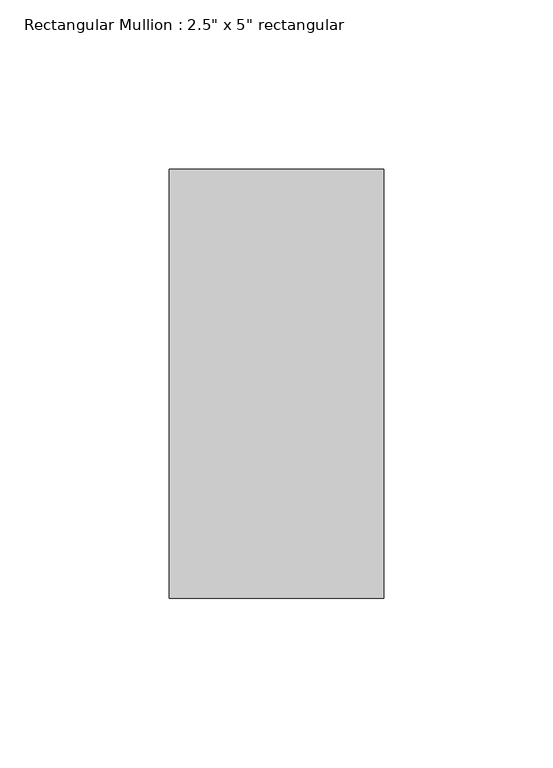
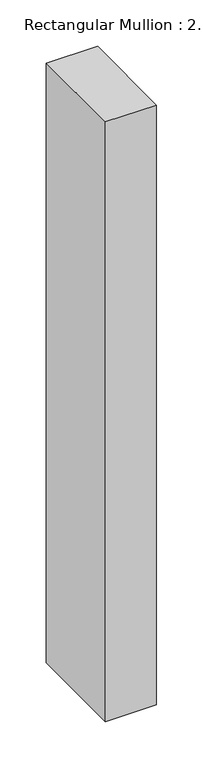
"""IFC4 building model written with IfcOpenShell, lengths in millimetres: member geometry."""

from ifc_helpers import new_model, si_unit, frame, origin, place, context, project, spatial, polyline, outline, extrude, source, transform, mapped, element, save


def member_58fda759(model_context):
    return source(origin(), model_context, "Body", "SweptSolid", [
        extrude(outline(polyline([(0.0, 63.5), (0.0, -63.5), (-63.5, -63.5), (-63.5, 63.5), (0.0, 63.5)])), frame((0.0, 0.0, -788.0989237), z_axis=(0.0, 0.0, 1.0), x_axis=(1.0, 0.0, 0.0)), (0.0, 0.0, 1.0), 788.0989237),
    ])


if __name__ == "__main__":
    model = new_model("IFC4")
    model_context = context("Model", 3, world=origin())
    ifc_project = project(units=[si_unit("LENGTHUNIT", "METRE", prefix="MILLI")], contexts=[model_context])
    site = spatial("IfcSite", under=ifc_project)
    building = spatial("IfcBuilding", under=site)
    placement = place(None, origin())
    member_shape = member_58fda759(model_context)
    element("IfcMember", 1, ObjectType="Rectangular Mullion : 2.5\" x 5\" rectangular", at=placement, inside=building, context=model_context, shape_type="MappedRepresentation", body=[
        mapped(member_shape, transform((0.0, 0.0, 0.0), x_axis=(1.0, 0.0, 0.0), y_axis=(0.0, 1.0, 0.0), z_axis=(0.0, 0.0, 1.0))),
    ])
    save(model, "model.ifc")

# Revit data of these elements
# Type "Rectangular Mullion : 2.5\" x 5\" rectangular"
#   built-in parameter 1007304 = 0.416667 (stored number, unit not read)
#   built-in parameter 1007301 = 0.104167 (stored number, unit not read)
#   built-in parameter 1007300 = 0.104167 (stored number, unit not read)
# Element 1 (IfcMember, "Rectangular Mullion : 2.5\" x 5\" rectangular")
#   Materials on its faces: "Aluminum"
# Materials
#   "Aluminum": class "Metal", colour RGB 247 247 247, transparency 0, Description = "Aluminum 6061", Cost = 0
